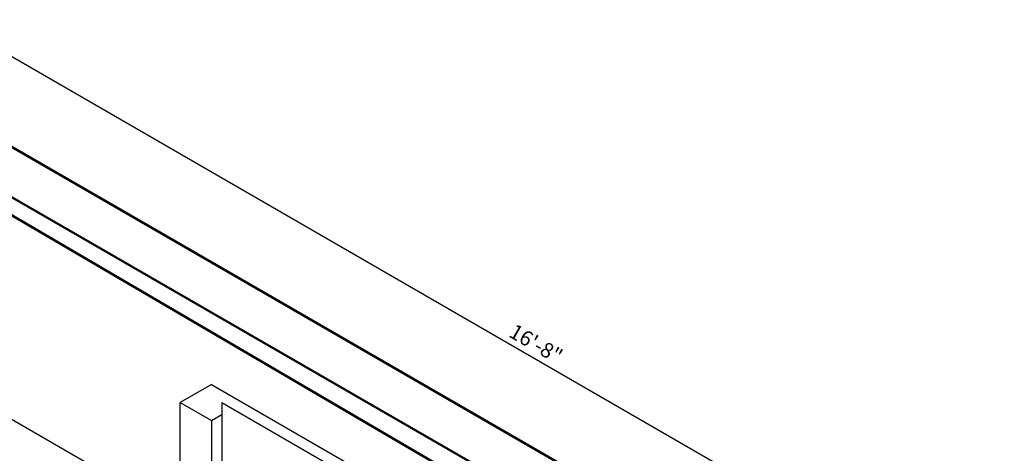
# Model space of a CAD drawing. Units: inches. Extents: x 5770 to 11891, y 3254 to 6808.
# Tile 14 of 15: x 5976 to 6140, y 3489 to 3561. Entities that reach past the tile are written whole.
import ezdxf

# ---------------------------------------------------------------- set-up
doc = ezdxf.new("R2010")
doc.units = ezdxf.units.IN
for name, color, linetype, lineweight in [('A-ANNO-DIMS', 2, 'Continuous', 18), ('A-FURN', 8, 'Continuous', 25), ('A-GLAZ', 4, 'Continuous', 25), ('A-WALL', 7, 'Continuous', 50)]:
    doc.layers.add(name, color=color, linetype=linetype, lineweight=lineweight)
doc.styles.get("Standard").update_dxf_attribs({"font": 'arial.ttf'})
doc.dimstyles.new('ISO-25', dxfattribs={"dimtxt": 2.5, "dimasz": 2.5, "dimexe": 1.25, "dimexo": 0.625, "dimtad": 1, "dimdec": 0, "dimlunit": 3, "dimtxsty": 'Standard', "dimcen": 2.5, "dimadec": 0, "dimazin": 0, "dimtfac": 1, "dimtdec": 0, "dimtmove": 0, "dimatfit": 3, "dimfxl": 1, "dimarcsym": 0})

# ---------------------------------------------------------------- blocks, each defined once
blk = doc.blocks.new('*D7')
at = {"layer": 'A-ANNO-DIMS', "color": 0, "lineweight": -2, "transparency": 16777216}
for p, q in [((5959.63, 3549.37), (5966.46, 3561.21)), ((5968, 3558.88), (6136.88, 3461.38)), ((6132.83, 3449.37), (6139.67, 3461.21))]:
    blk.add_line(p, q, dxfattribs=at)
at = {"layer": 'A-ANNO-DIMS', "color": 0, "transparency": 16777216}
for points in [[(5968.21, 3559.24), (5967.79, 3558.51), (5965.84, 3560.13)], [(6137.08, 3461.74), (6136.67, 3461.01), (6139.04, 3460.13)]]:
    blk.add_solid(points, dxfattribs=at)
at = {"layer": 'Defpoints', "color": 0, "transparency": 16777216}
for p in [(5959.31, 3548.83), (6139.04, 3460.13), (6132.52, 3448.83)]:
    blk.add_point(p, dxfattribs=at)
at = {"layer": 'A-ANNO-DIMS', "color": 0, "transparency": 16777216, "insert": (6061.62, 3507.02), "char_height": 2.5, "attachment_point": 5, "rotation": 330}
blk.add_mtext('16\'-8"', dxfattribs=at)

msp = doc.modelspace()

# ---------------------------------------------------------------- linework, layer by layer
at = {"layer": 'A-FURN'}
for p, q in [((6002.6, 3455.52), (6002.6, 3497.52)), ((5974.02, 3495.06), (6002.6, 3478.56))]:
    msp.add_line(p, q, dxfattribs=at)
at = {"layer": 'A-GLAZ'}
for p, q in [((6007.8, 3500.52), (6002.6, 3497.52)), ((6007.8, 3500.52), (6049.36, 3476.52)), ((6002.6, 3497.52), (6007.8, 3494.52)), ((6009.53, 3497.52), (6047.63, 3475.52)), ((6009.53, 3497.52), (6009.53, 3459.52)), ((6007.8, 3494.52), (6009.53, 3495.52)), ((6007.8, 3494.52), (6007.8, 3458.52))]:
    msp.add_line(p, q, dxfattribs=at)
at = {"layer": 'A-WALL'}
for p, q in [((5959.31, 3548.83), (6132.52, 3448.83)), ((5959.31, 3540.51), (6115.24, 3450.48)), ((5974.02, 3529.02), (6111.68, 3448.43))]:
    msp.add_line(p, q, dxfattribs=at)

# ---------------------------------------------------------------- dimensions: what is measured, and where the dimension line sits
at = {"layer": 'A-ANNO-DIMS'}
dim = msp.add_linear_dim(base=(6139.04, 3460.13), p1=(5959.31, 3548.83), p2=(6132.52, 3448.83), angle=330, dimstyle='ISO-25', override={"dimclrd": 0, "dimclre": 0, "dimclrt": 0}, dxfattribs=at)
dim.commit()
dim.dimension.update_dxf_attribs({"geometry": '*D7', "text_midpoint": (6060.67, 3505.37), "dimtype": 161})

doc.saveas('drawing.dxf')
